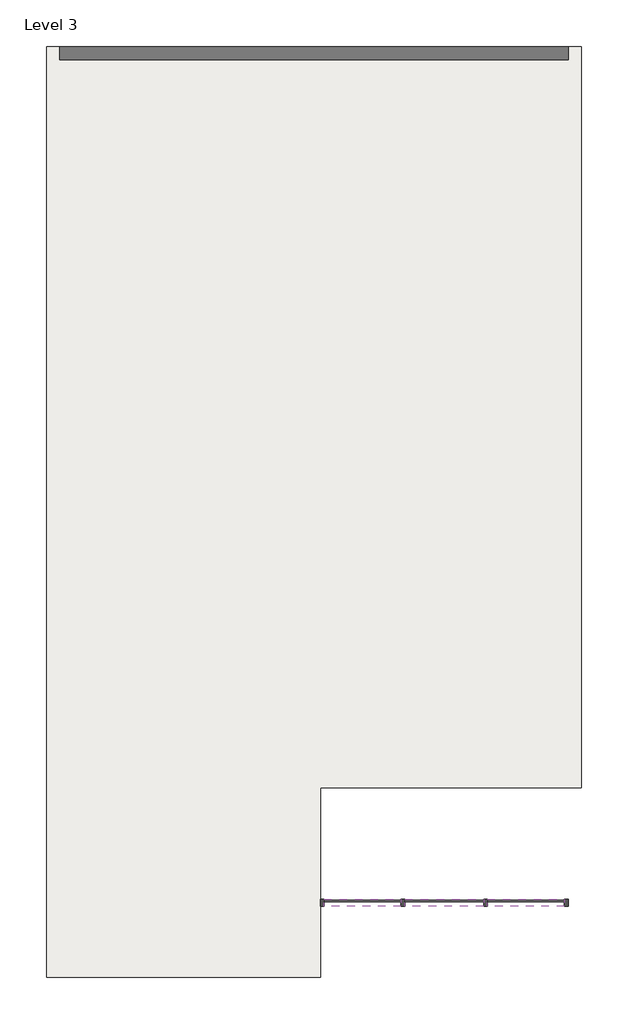
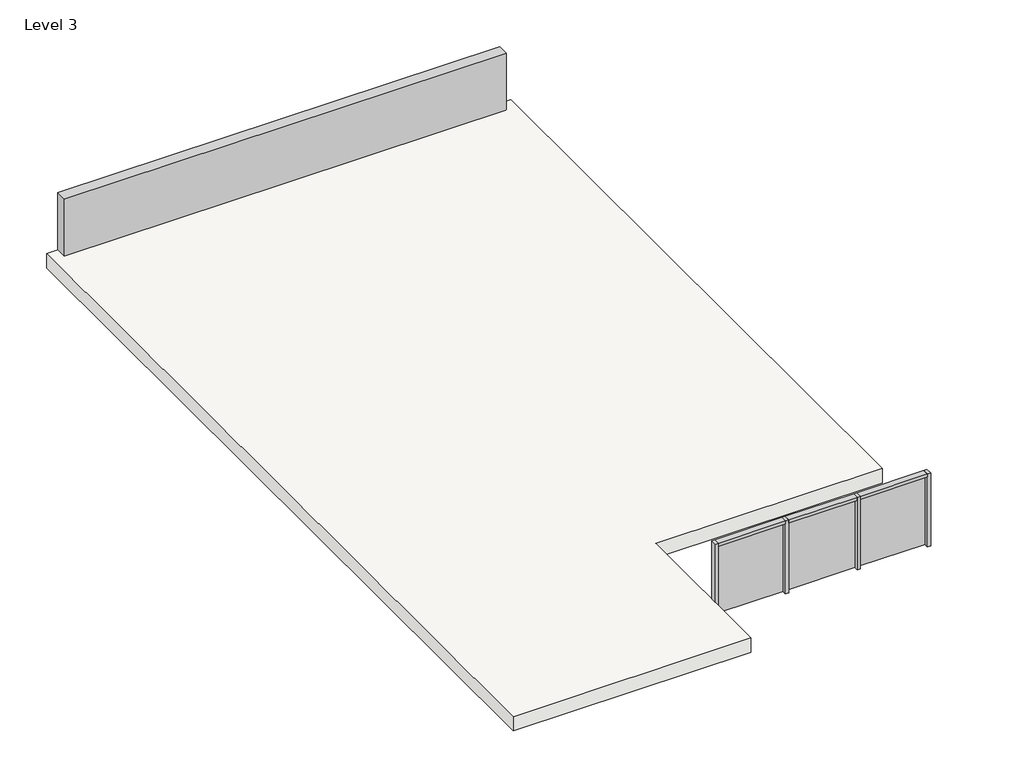
# One storey: 7 members, 3 plates, 1 proxy, 1 roof.
"""IFC4 building model written with IfcOpenShell, lengths in millimetres."""

from ifc_helpers import new_model, si_unit, frame, origin, place, context, project, spatial, polyline, outline, extrude, transform, mapped, element, save
from components import generic_models_4_generic_models_4_25668e5e, member_20eb5ac3, member_e1cf819f, member_0499d444, member_8c7debe4, system_panel_glazed_1570095f, system_panel_glazed_0767085a

model = new_model("IFC4")

# Units and contexts
model_context = context("Model", 3, world=origin())
ifc_project = project(units=[si_unit("LENGTHUNIT", "METRE", prefix="MILLI")], contexts=[model_context])

# Site, building, storey
site = spatial("IfcSite", under=ifc_project)
building = spatial("IfcBuilding", under=site)
storey = spatial("IfcBuildingStorey", under=building, Name="Level 3", Elevation=6096.0)

# Proxy
placement = place(None, origin())
generic_models_4_generic_models_4_shape = generic_models_4_generic_models_4_25668e5e(model_context)
element("IfcBuildingElementProxy", 1, Name="Generic Models 4 : Generic Models 4", ObjectType="Generic Models 4 : Generic Models 4", at=placement, inside=storey, context=model_context, shape_type="MappedRepresentation", body=[
    mapped(generic_models_4_generic_models_4_shape, transform((0.0, 0.0, 0.0), x_axis=(1.0, 0.0, 0.0), y_axis=(0.0, 1.0, 0.0), z_axis=(0.0, 0.0, 1.0))),
])

# Members
member_shape = member_20eb5ac3(model_context)
element("IfcMember", 2, ObjectType="Rectangular Mullion : 2.5\" x 5\" rectangular", at=placement, inside=storey, context=model_context, shape_type="MappedRepresentation", body=[
    mapped(member_shape, transform((-13876.3661422, -9510.8644962, 7646.242764), x_axis=(0.0, 0.0, 1.0), y_axis=(0.0, -1.0, 0.0), z_axis=(1.0, 0.0, 0.0))),
])
element("IfcMember", 3, ObjectType="Rectangular Mullion : 2.5\" x 5\" rectangular", at=placement, inside=storey, context=model_context, shape_type="MappedRepresentation", body=[
    mapped(member_shape, transform((-11012.5161422, -9510.8644962, 7646.242764), x_axis=(0.0, 0.0, 1.0), y_axis=(0.0, -1.0, 0.0), z_axis=(1.0, 0.0, 0.0))),
])
member_2_shape = member_e1cf819f(model_context)
element("IfcMember", 4, ObjectType="Rectangular Mullion : 2.5\" x 5\" rectangular", at=placement, inside=storey, context=model_context, shape_type="MappedRepresentation", body=[
    mapped(member_2_shape, transform((-12428.5661422, -9510.8644962, 7646.242764), x_axis=(0.0, 0.0, 1.0), y_axis=(0.0, -1.0, 0.0), z_axis=(1.0, 0.0, 0.0))),
])
member_3_shape = member_0499d444(model_context)
element("IfcMember", 5, ObjectType="Rectangular Mullion : 2.5\" x 5\" rectangular", at=placement, inside=storey, context=model_context, shape_type="MappedRepresentation", body=[
    mapped(member_3_shape, transform((-15292.4161422, -9510.8644962, 7646.242764), x_axis=(-1.0, 0.0, 0.0), y_axis=(0.0, -1.0, 0.0), z_axis=(0.0, 0.0, 1.0))),
])
member_4_shape = member_8c7debe4(model_context)
element("IfcMember", 6, ObjectType="Rectangular Mullion : 2.5\" x 5\" rectangular", at=placement, inside=storey, context=model_context, shape_type="MappedRepresentation", body=[
    mapped(member_4_shape, transform((-13844.6161422, -9510.8644962, 6096.0), x_axis=(1.0, 0.0, 0.0), y_axis=(0.0, -1.0, 0.0), z_axis=(0.0, 0.0, -1.0))),
])
element("IfcMember", 7, ObjectType="Rectangular Mullion : 2.5\" x 5\" rectangular", at=placement, inside=storey, context=model_context, shape_type="MappedRepresentation", body=[
    mapped(member_4_shape, transform((-12396.8161422, -9510.8644962, 6096.0), x_axis=(1.0, 0.0, 0.0), y_axis=(0.0, -1.0, 0.0), z_axis=(0.0, 0.0, -1.0))),
])
element("IfcMember", 8, ObjectType="Rectangular Mullion : 2.5\" x 5\" rectangular", at=placement, inside=storey, context=model_context, shape_type="MappedRepresentation", body=[
    mapped(member_3_shape, transform((-10949.0161422, -9510.8644962, 6096.0), x_axis=(1.0, 0.0, 0.0), y_axis=(0.0, -1.0, 0.0), z_axis=(0.0, 0.0, -1.0))),
])

# Plates
system_panel_glazed_shape = system_panel_glazed_1570095f(model_context)
element("IfcPlate", 9, ObjectType="System Panel : Glazed", at=placement, inside=storey, context=model_context, shape_type="MappedRepresentation", body=[
    mapped(system_panel_glazed_shape, transform((-14552.6411422, -9510.8644962, 6096.0), x_axis=(1.0, 0.0, 0.0), y_axis=(0.0, 1.0, 0.0), z_axis=(0.0, 0.0, 1.0))),
])
element("IfcPlate", 10, ObjectType="System Panel : Glazed", at=placement, inside=storey, context=model_context, shape_type="MappedRepresentation", body=[
    mapped(system_panel_glazed_shape, transform((-11688.7911422, -9510.8644962, 6096.0), x_axis=(1.0, 0.0, 0.0), y_axis=(0.0, 1.0, 0.0), z_axis=(0.0, 0.0, 1.0))),
])
system_panel_glazed_2_shape = system_panel_glazed_0767085a(model_context)
element("IfcPlate", 11, ObjectType="System Panel : Glazed", at=placement, inside=storey, context=model_context, shape_type="MappedRepresentation", body=[
    mapped(system_panel_glazed_2_shape, transform((-13120.7161422, -9510.8644962, 6096.0), x_axis=(1.0, 0.0, 0.0), y_axis=(0.0, 1.0, 0.0), z_axis=(0.0, 0.0, 1.0))),
])

# Roof
element("IfcRoof", 12, ObjectType="Generic - 12\"", at=placement, inside=storey, context=model_context, shape_type="SweptSolid", body=[
    extrude(outline(polyline([(-20093.0161422, 5487.8132242), (-10720.4161422, 5487.8132242), (-10720.4161422, -7491.5867758), (-15292.4161422, -7491.5867758), (-15292.4161422, -10818.9867758), (-20093.0161422, -10818.9867758), (-20093.0161422, 5487.8132242)])), frame((0.0, 0.0, 6096.0), z_axis=(0.0, 0.0, 1.0), x_axis=(1.0, 0.0, 0.0)), (0.0, 0.0, 1.0), 304.8),
])

save(model, "model.ifc")

# Revit data of these elements
# Type "Rectangular Mullion : 2.5\" x 5\" rectangular"
#   built-in parameter 1007304 = 0.416667 (stored number, unit not read)
#   built-in parameter 1007301 = 0.104167 (stored number, unit not read)
#   built-in parameter 1007300 = 0.104167 (stored number, unit not read)
# Type "System Panel : Glazed"
#   Construction Type Id = "GSP4R"
#   Analytic Construction = "1/8 in Pilkington single glazing"
#   Visual Light Transmittance = 0.9
#   Solar Heat Gain Coefficient = 0.86
#   Heat Transfer Coefficient (U) = 1.18115 BTU/(h·ft²·°F)
#   Define Thermal Properties by = 1
# Type "Generic - 12\""
#   Assembly Code = "B1020"
#   Layers, outside or top first: 1' - 0" no material (function 1)
# Element 1 (IfcBuildingElementProxy, "Generic Models 4 : Generic Models 4")
#   Phase Created = New Construction
# Elements 2, 3, 4, 5, 6, 7, 8 (IfcMember, "Rectangular Mullion : 2.5\" x 5\" rectangular")
#   Phase Created = New Construction
#   Materials on its faces: "Aluminum"
# Elements 9, 10, 11 (IfcPlate, "System Panel : Glazed")
#   Phase Created = New Construction
#   Materials on its faces: "Glass"
# Element 12 (IfcRoof, "Generic - 12\"")
#   built-in parameter 1001705 = 21 (stored number, unit not read)
#   built-in parameter 1001710 = 33615
#   Phase Created = New Construction
#   Materials on its faces: "Default Roof"
# Materials
#   "Aluminum": class "Metal", colour RGB 247 247 247, transparency 0, Description = "Aluminum 6061", Cost = 0
#   "Glass": class "Glass", colour RGB 0 128 192, transparency 0.75, Description = "Soda Lime Glass", Cost = 0
#   "Default Roof": colour RGB 88 101 114, transparency 0, Cost = 0
